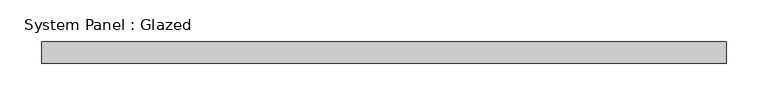
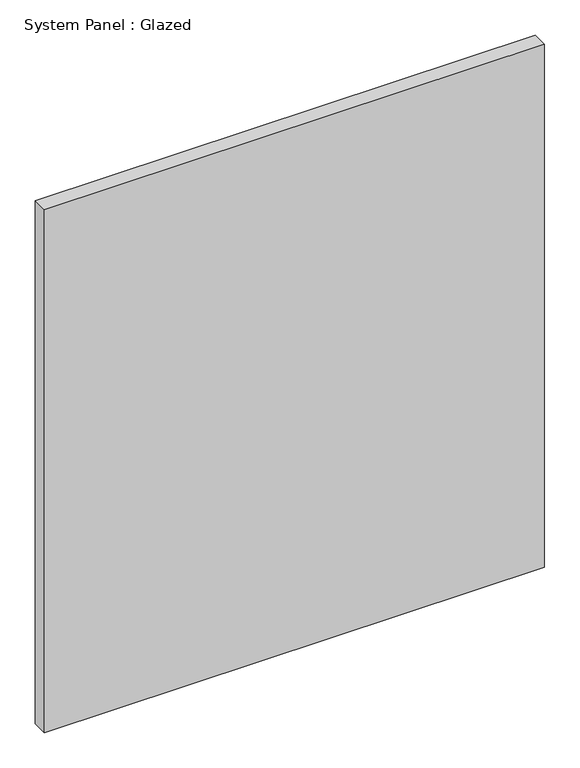
"""IFC4 building model written with IfcOpenShell, lengths in millimetres: plate geometry, System Panel : Glazed."""

from ifc_helpers import new_model, si_unit, origin, origin_with_axes, place, context, project, spatial, polyline, outline, extrude, source, transform, mapped, element, save


def system_panel_glazed_dab0583a(model_context):
    return source(origin(), model_context, "Body", "SweptSolid", [
        extrude(outline(polyline([(409.575, 19.05), (-409.575, 19.05), (-409.575, 44.45), (409.575, 44.45), (409.575, 19.05)])), origin_with_axes(), (0.0, 0.0, 1.0), 905.7522263),
    ])


if __name__ == "__main__":
    model = new_model("IFC4")
    model_context = context("Model", 3, world=origin())
    ifc_project = project(units=[si_unit("LENGTHUNIT", "METRE", prefix="MILLI")], contexts=[model_context])
    site = spatial("IfcSite", under=ifc_project)
    building = spatial("IfcBuilding", under=site)
    placement = place(None, origin())
    system_panel_glazed_shape = system_panel_glazed_dab0583a(model_context)
    element("IfcPlate", 1, ObjectType="System Panel : Glazed", at=placement, inside=building, context=model_context, shape_type="MappedRepresentation", body=[
        mapped(system_panel_glazed_shape, transform((0.0, 0.0, 0.0), x_axis=(1.0, 0.0, 0.0), y_axis=(0.0, 1.0, 0.0), z_axis=(0.0, 0.0, 1.0))),
    ])
    save(model, "model.ifc")

# Revit data of these elements
# Type "System Panel : Glazed"
#   Construction Type Id = "GSP4R"
#   Analytic Construction = "1/8 in Pilkington single glazing"
#   Visual Light Transmittance = 0.9
#   Solar Heat Gain Coefficient = 0.86
#   Heat Transfer Coefficient (U) = 1.18115 BTU/(h·ft²·°F)
#   Define Thermal Properties by = 1
# Element 1 (IfcPlate, "System Panel : Glazed")
#   Materials on its faces: "Glass"
# Materials
#   "Glass": class "Glass", colour RGB 0 128 192, transparency 0.75, Description = "Soda Lime Glass", Cost = 0
